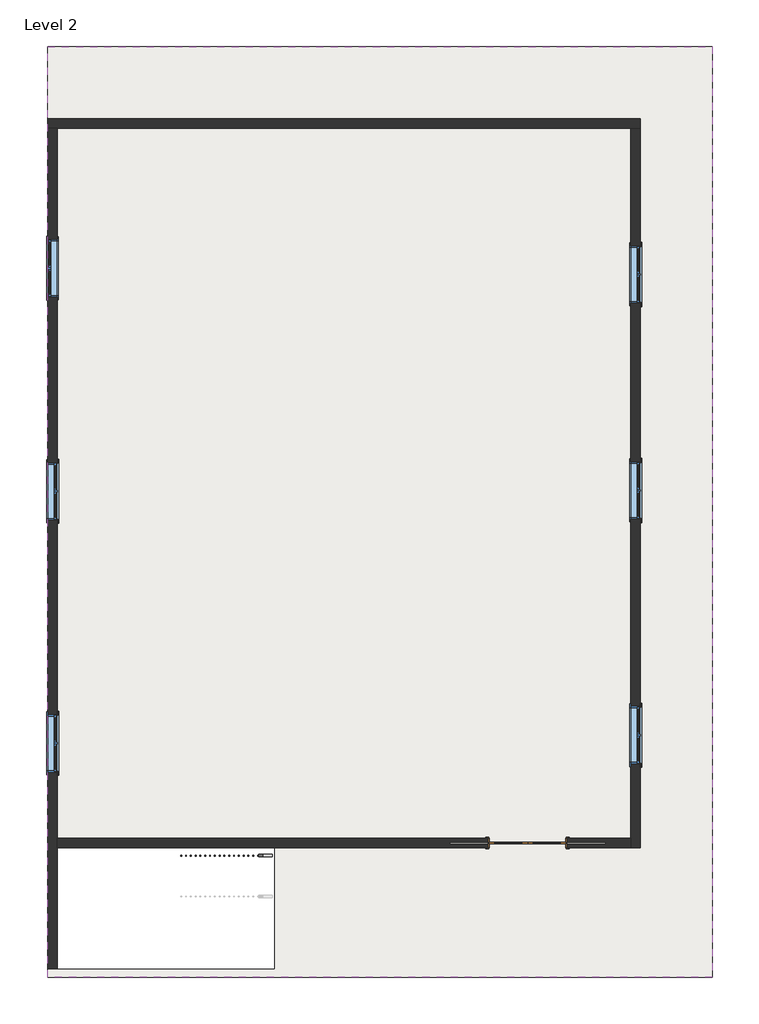
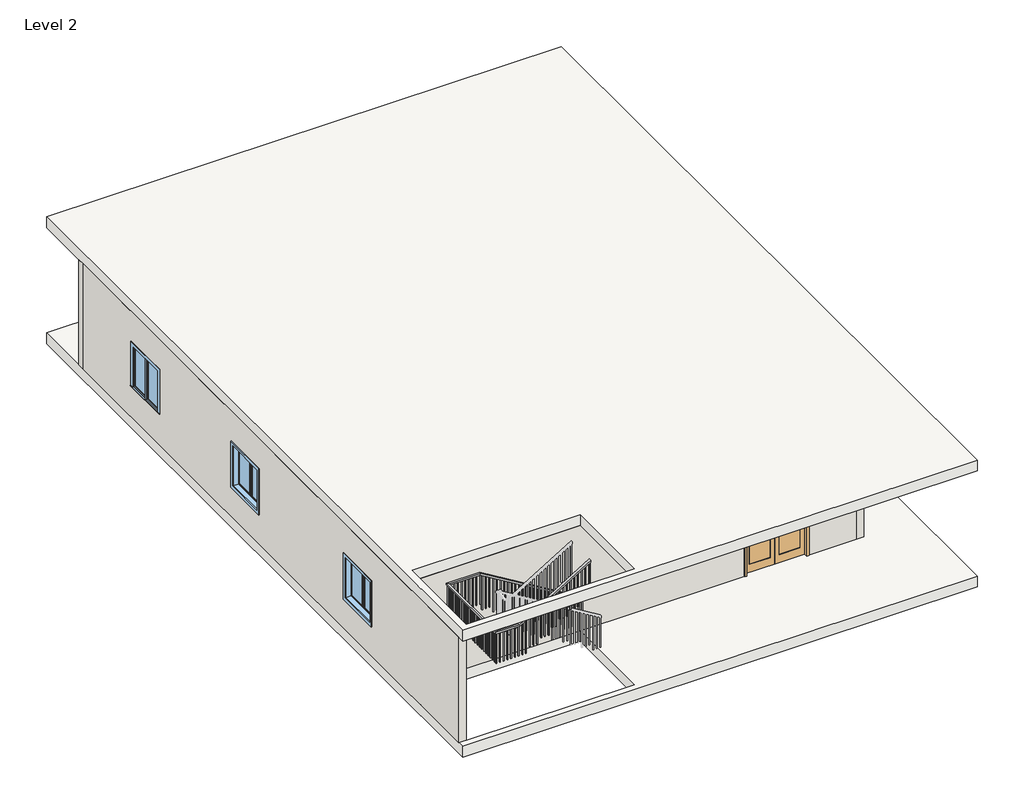
# One storey, part 1 of 2: 6 windows, 4 walls, 2 slabs, 1 door, 1 railing.
"""IFC4 building model written with IfcOpenShell, lengths in millimetres."""

from ifc_helpers import new_model, si_unit, frame, origin, place, context, project, spatial, polyline, outline, extrude, faceted_brep, transform, mapped, element, save
from components import door_18a53484, window_0862ab64

model = new_model("IFC4")

# Units and contexts
model_context = context("Model", 3, world=origin())
ifc_project = project(units=[si_unit("LENGTHUNIT", "METRE", prefix="MILLI")], contexts=[model_context])

# Site, building, storey
site = spatial("IfcSite", under=ifc_project)
building = spatial("IfcBuilding", under=site)
storey = spatial("IfcBuildingStorey", under=building, Name="Level 2", Elevation=3048.0)

# Door
placement = place(None, origin())
door_shape = door_18a53484(model_context)
element("IfcDoor", 1, ObjectType="Door-Interior-Double-Pocket-2_Panel-Wood : 64\" x 80\"", at=placement, inside=storey, context=model_context, shape_type="MappedRepresentation", body=[
    mapped(door_shape, transform((-1633.6127533, -5879.8242744, 3048.0), x_axis=(1.0, 0.0, 0.0), y_axis=(0.0, 1.0, 0.0), z_axis=(0.0, 0.0, 1.0))),
])

# Railing
element("IfcRailing", 2, ObjectType="Handrail - Rectangular", at=placement, inside=storey, context=model_context, shape_type="SolidModel", body=[
    faceted_brep([(-7036.5382419, -6171.9242744, 4131.7333333), (-7036.5382419, -6171.9242744, 4072.3318731), (-7036.5382419, -6121.1242744, 4072.3318731), (-7036.5382419, -6121.1242744, 4131.7333333), (-9830.5382419, -6171.9242744, 5825.0666667), (-9844.7306513, -6171.9242744, 5774.2666667), (-9844.7306513, -6121.1242744, 5774.2666667), (-9830.5382419, -6121.1242744, 5825.0666667), (-10694.1382419, -6171.9242744, 5825.0666667), (-10694.1382419, -6171.9242744, 5774.2666667), (-10744.9382419, -6121.1242744, 5774.2666667), (-10744.9382419, -6121.1242744, 5825.0666667), (-10694.1382419, -8420.4243151, 5825.0666667), (-10694.1382419, -8420.4243151, 5774.2666667), (-10744.9382419, -8471.2243151, 5774.2666667), (-10744.9382419, -8471.2243151, 5825.0666667), (-10109.9382419, -8420.4243151, 5825.0666667), (-10095.7458325, -8420.4243151, 5774.2666667), (-10095.7458325, -8471.2243151, 5774.2666667), (-10109.9382419, -8471.2243151, 5825.0666667), (-8154.1382419, -8420.4243151, 7010.4), (-8154.1382419, -8471.2243151, 7010.4), (-8154.1382419, -8471.2243151, 6950.9985397), (-8154.1382419, -8420.4243151, 6950.9985397)], [[[0, 1, 2, 3]], [[1, 0, 4, 5]], [[2, 1, 5, 6]], [[3, 2, 6, 7]], [[0, 3, 7, 4]], [[5, 4, 8, 9]], [[6, 5, 9, 10]], [[7, 6, 10, 11]], [[4, 7, 11, 8]], [[9, 8, 12, 13]], [[10, 9, 13, 14]], [[11, 10, 14, 15]], [[8, 11, 15, 12]], [[13, 12, 16, 17]], [[14, 13, 17, 18]], [[15, 14, 18, 19]], [[12, 15, 19, 16]], [[20, 21, 22, 23]], [[17, 16, 20, 23]], [[18, 17, 23, 22]], [[19, 18, 22, 21]], [[16, 19, 21, 20]]]),
    extrude(outline(polyline([(6941.3773276, -8170.0132419), (6929.8318731, -8189.0632419), (5926.6666667, -8189.0632419), (5926.6666667, -8170.0132419), (6941.3773276, -8170.0132419)])), frame((0.0, -8455.3493151, 0.0), z_axis=(0.0, 1.0, 0.0), x_axis=(0.0, 0.0, 1.0)), (0.0, 0.0, 1.0), 19.05),
    extrude(outline(polyline([(6879.80157, -8271.6132419), (6868.2561155, -8290.6632419), (5926.6666667, -8290.6632419), (5926.6666667, -8271.6132419), (6879.80157, -8271.6132419)])), frame((0.0, -8455.3493151, 0.0), z_axis=(0.0, 1.0, 0.0), x_axis=(0.0, 0.0, 1.0)), (0.0, 0.0, 1.0), 19.05),
    extrude(outline(polyline([(6818.2258125, -8373.2132419), (6806.6803579, -8392.2632419), (5926.6666667, -8392.2632419), (5926.6666667, -8373.2132419), (6818.2258125, -8373.2132419)])), frame((0.0, -8455.3493151, 0.0), z_axis=(0.0, 1.0, 0.0), x_axis=(0.0, 0.0, 1.0)), (0.0, 0.0, 1.0), 19.05),
    extrude(outline(polyline([(6756.6500549, -8474.8132419), (6745.1046004, -8493.8632419), (5757.3333333, -8493.8632419), (5757.3333333, -8474.8132419), (6756.6500549, -8474.8132419)])), frame((0.0, -8455.3493151, 0.0), z_axis=(0.0, 1.0, 0.0), x_axis=(0.0, 0.0, 1.0)), (0.0, 0.0, 1.0), 19.05),
    extrude(outline(polyline([(6695.0742973, -8576.4132419), (6683.5288428, -8595.4632419), (5757.3333333, -8595.4632419), (5757.3333333, -8576.4132419), (6695.0742973, -8576.4132419)])), frame((0.0, -8455.3493151, 0.0), z_axis=(0.0, 1.0, 0.0), x_axis=(0.0, 0.0, 1.0)), (0.0, 0.0, 1.0), 19.05),
    extrude(outline(polyline([(6633.4985397, -8678.0132419), (6621.9530852, -8697.0632419), (5757.3333333, -8697.0632419), (5757.3333333, -8678.0132419), (6633.4985397, -8678.0132419)])), frame((0.0, -8455.3493151, 0.0), z_axis=(0.0, 1.0, 0.0), x_axis=(0.0, 0.0, 1.0)), (0.0, 0.0, 1.0), 19.05),
    extrude(outline(polyline([(6571.9227822, -8779.6132419), (6560.3773276, -8798.6632419), (5588.0, -8798.6632419), (5588.0, -8779.6132419), (6571.9227822, -8779.6132419)])), frame((0.0, -8455.3493151, 0.0), z_axis=(0.0, 1.0, 0.0), x_axis=(0.0, 0.0, 1.0)), (0.0, 0.0, 1.0), 19.05),
    extrude(outline(polyline([(6510.3470246, -8881.2132419), (6498.80157, -8900.2632419), (5588.0, -8900.2632419), (5588.0, -8881.2132419), (6510.3470246, -8881.2132419)])), frame((0.0, -8455.3493151, 0.0), z_axis=(0.0, 1.0, 0.0), x_axis=(0.0, 0.0, 1.0)), (0.0, 0.0, 1.0), 19.05),
    extrude(outline(polyline([(6448.771267, -8982.8132419), (6437.2258125, -9001.8632419), (5588.0, -9001.8632419), (5588.0, -8982.8132419), (6448.771267, -8982.8132419)])), frame((0.0, -8455.3493151, 0.0), z_axis=(0.0, 1.0, 0.0), x_axis=(0.0, 0.0, 1.0)), (0.0, 0.0, 1.0), 19.05),
    extrude(outline(polyline([(6387.1955094, -9084.4132419), (6375.6500549, -9103.4632419), (5418.6666667, -9103.4632419), (5418.6666667, -9084.4132419), (6387.1955094, -9084.4132419)])), frame((0.0, -8455.3493151, 0.0), z_axis=(0.0, 1.0, 0.0), x_axis=(0.0, 0.0, 1.0)), (0.0, 0.0, 1.0), 19.05),
    extrude(outline(polyline([(6325.6197519, -9186.0132419), (6314.0742973, -9205.0632419), (5418.6666667, -9205.0632419), (5418.6666667, -9186.0132419), (6325.6197519, -9186.0132419)])), frame((0.0, -8455.3493151, 0.0), z_axis=(0.0, 1.0, 0.0), x_axis=(0.0, 0.0, 1.0)), (0.0, 0.0, 1.0), 19.05),
    extrude(outline(polyline([(6264.0439943, -9287.6132419), (6252.4985397, -9306.6632419), (5249.3333333, -9306.6632419), (5249.3333333, -9287.6132419), (6264.0439943, -9287.6132419)])), frame((0.0, -8455.3493151, 0.0), z_axis=(0.0, 1.0, 0.0), x_axis=(0.0, 0.0, 1.0)), (0.0, 0.0, 1.0), 19.05),
    extrude(outline(polyline([(6202.4682367, -9389.2132419), (6190.9227822, -9408.2632419), (5249.3333333, -9408.2632419), (5249.3333333, -9389.2132419), (6202.4682367, -9389.2132419)])), frame((0.0, -8455.3493151, 0.0), z_axis=(0.0, 1.0, 0.0), x_axis=(0.0, 0.0, 1.0)), (0.0, 0.0, 1.0), 19.05),
    extrude(outline(polyline([(6140.8924791, -9490.8132419), (6129.3470246, -9509.8632419), (5249.3333333, -9509.8632419), (5249.3333333, -9490.8132419), (6140.8924791, -9490.8132419)])), frame((0.0, -8455.3493151, 0.0), z_axis=(0.0, 1.0, 0.0), x_axis=(0.0, 0.0, 1.0)), (0.0, 0.0, 1.0), 19.05),
    extrude(outline(polyline([(6079.3167216, -9592.4132419), (6067.771267, -9611.4632419), (5080.0, -9611.4632419), (5080.0, -9592.4132419), (6079.3167216, -9592.4132419)])), frame((0.0, -8455.3493151, 0.0), z_axis=(0.0, 1.0, 0.0), x_axis=(0.0, 0.0, 1.0)), (0.0, 0.0, 1.0), 19.05),
    extrude(outline(polyline([(6017.740964, -9694.0132419), (6006.1955094, -9713.0632419), (5080.0, -9713.0632419), (5080.0, -9694.0132419), (6017.740964, -9694.0132419)])), frame((0.0, -8455.3493151, 0.0), z_axis=(0.0, 1.0, 0.0), x_axis=(0.0, 0.0, 1.0)), (0.0, 0.0, 1.0), 19.05),
    extrude(outline(polyline([(5956.1652064, -9795.6132419), (5944.6197519, -9814.6632419), (5080.0, -9814.6632419), (5080.0, -9795.6132419), (5956.1652064, -9795.6132419)])), frame((0.0, -8455.3493151, 0.0), z_axis=(0.0, 1.0, 0.0), x_axis=(0.0, 0.0, 1.0)), (0.0, 0.0, 1.0), 19.05),
    extrude(outline(polyline([(5894.5894488, -9897.2132419), (5883.0439943, -9916.2632419), (4910.6666667, -9916.2632419), (4910.6666667, -9897.2132419), (5894.5894488, -9897.2132419)])), frame((0.0, -8455.3493151, 0.0), z_axis=(0.0, 1.0, 0.0), x_axis=(0.0, 0.0, 1.0)), (0.0, 0.0, 1.0), 19.05),
    extrude(outline(polyline([(5833.0136913, -9998.8132419), (5821.4682367, -10017.8632419), (4910.6666667, -10017.8632419), (4910.6666667, -9998.8132419), (5833.0136913, -9998.8132419)])), frame((0.0, -8455.3493151, 0.0), z_axis=(0.0, 1.0, 0.0), x_axis=(0.0, 0.0, 1.0)), (0.0, 0.0, 1.0), 19.05),
    extrude(outline(polyline([(-10221.0632419, -8455.3493151), (-10221.0632419, -8436.2993151), (-10202.0132419, -8436.2993151), (-10202.0132419, -8455.3493151), (-10221.0632419, -8455.3493151)])), frame((0.0, 0.0, 4910.6666667), z_axis=(0.0, 0.0, 1.0), x_axis=(1.0, 0.0, 0.0)), (0.0, 0.0, 1.0), 863.6),
    extrude(outline(polyline([(-10322.6632419, -8455.3493151), (-10322.6632419, -8436.2993151), (-10303.6132419, -8436.2993151), (-10303.6132419, -8455.3493151), (-10322.6632419, -8455.3493151)])), frame((0.0, 0.0, 4910.6666667), z_axis=(0.0, 0.0, 1.0), x_axis=(1.0, 0.0, 0.0)), (0.0, 0.0, 1.0), 863.6),
    extrude(outline(polyline([(-10424.2632419, -8455.3493151), (-10424.2632419, -8436.2993151), (-10405.2132419, -8436.2993151), (-10405.2132419, -8455.3493151), (-10424.2632419, -8455.3493151)])), frame((0.0, 0.0, 4910.6666667), z_axis=(0.0, 0.0, 1.0), x_axis=(1.0, 0.0, 0.0)), (0.0, 0.0, 1.0), 863.6),
    extrude(outline(polyline([(-10525.8632419, -8455.3493151), (-10525.8632419, -8436.2993151), (-10506.8132419, -8436.2993151), (-10506.8132419, -8455.3493151), (-10525.8632419, -8455.3493151)])), frame((0.0, 0.0, 4910.6666667), z_axis=(0.0, 0.0, 1.0), x_axis=(1.0, 0.0, 0.0)), (0.0, 0.0, 1.0), 863.6),
    extrude(outline(polyline([(-10627.4632419, -8455.3493151), (-10627.4632419, -8436.2993151), (-10608.4132419, -8436.2993151), (-10608.4132419, -8455.3493151), (-10627.4632419, -8455.3493151)])), frame((0.0, 0.0, 4910.6666667), z_axis=(0.0, 0.0, 1.0), x_axis=(1.0, 0.0, 0.0)), (0.0, 0.0, 1.0), 863.6),
    extrude(outline(polyline([(-10729.0632419, -8372.1992744), (-10710.0132419, -8372.1992744), (-10710.0132419, -8391.2492744), (-10729.0632419, -8391.2492744), (-10729.0632419, -8372.1992744)])), frame((0.0, 0.0, 4910.6666667), z_axis=(0.0, 0.0, 1.0), x_axis=(1.0, 0.0, 0.0)), (0.0, 0.0, 1.0), 863.6),
    extrude(outline(polyline([(-10729.0632419, -8270.5992744), (-10710.0132419, -8270.5992744), (-10710.0132419, -8289.6492744), (-10729.0632419, -8289.6492744), (-10729.0632419, -8270.5992744)])), frame((0.0, 0.0, 4910.6666667), z_axis=(0.0, 0.0, 1.0), x_axis=(1.0, 0.0, 0.0)), (0.0, 0.0, 1.0), 863.6),
    extrude(outline(polyline([(-10729.0632419, -8168.9992744), (-10710.0132419, -8168.9992744), (-10710.0132419, -8188.0492744), (-10729.0632419, -8188.0492744), (-10729.0632419, -8168.9992744)])), frame((0.0, 0.0, 4910.6666667), z_axis=(0.0, 0.0, 1.0), x_axis=(1.0, 0.0, 0.0)), (0.0, 0.0, 1.0), 863.6),
    extrude(outline(polyline([(-10729.0632419, -8067.3992744), (-10710.0132419, -8067.3992744), (-10710.0132419, -8086.4492744), (-10729.0632419, -8086.4492744), (-10729.0632419, -8067.3992744)])), frame((0.0, 0.0, 4910.6666667), z_axis=(0.0, 0.0, 1.0), x_axis=(1.0, 0.0, 0.0)), (0.0, 0.0, 1.0), 863.6),
    extrude(outline(polyline([(-10729.0632419, -7965.7992744), (-10710.0132419, -7965.7992744), (-10710.0132419, -7984.8492744), (-10729.0632419, -7984.8492744), (-10729.0632419, -7965.7992744)])), frame((0.0, 0.0, 4910.6666667), z_axis=(0.0, 0.0, 1.0), x_axis=(1.0, 0.0, 0.0)), (0.0, 0.0, 1.0), 863.6),
    extrude(outline(polyline([(-10729.0632419, -7864.1992744), (-10710.0132419, -7864.1992744), (-10710.0132419, -7883.2492744), (-10729.0632419, -7883.2492744), (-10729.0632419, -7864.1992744)])), frame((0.0, 0.0, 4910.6666667), z_axis=(0.0, 0.0, 1.0), x_axis=(1.0, 0.0, 0.0)), (0.0, 0.0, 1.0), 863.6),
    extrude(outline(polyline([(-10729.0632419, -7762.5992744), (-10710.0132419, -7762.5992744), (-10710.0132419, -7781.6492744), (-10729.0632419, -7781.6492744), (-10729.0632419, -7762.5992744)])), frame((0.0, 0.0, 4910.6666667), z_axis=(0.0, 0.0, 1.0), x_axis=(1.0, 0.0, 0.0)), (0.0, 0.0, 1.0), 863.6),
    extrude(outline(polyline([(-10729.0632419, -7660.9992744), (-10710.0132419, -7660.9992744), (-10710.0132419, -7680.0492744), (-10729.0632419, -7680.0492744), (-10729.0632419, -7660.9992744)])), frame((0.0, 0.0, 4910.6666667), z_axis=(0.0, 0.0, 1.0), x_axis=(1.0, 0.0, 0.0)), (0.0, 0.0, 1.0), 863.6),
    extrude(outline(polyline([(-10729.0632419, -7559.3992744), (-10710.0132419, -7559.3992744), (-10710.0132419, -7578.4492744), (-10729.0632419, -7578.4492744), (-10729.0632419, -7559.3992744)])), frame((0.0, 0.0, 4910.6666667), z_axis=(0.0, 0.0, 1.0), x_axis=(1.0, 0.0, 0.0)), (0.0, 0.0, 1.0), 863.6),
    extrude(outline(polyline([(-10729.0632419, -7457.7992744), (-10710.0132419, -7457.7992744), (-10710.0132419, -7476.8492744), (-10729.0632419, -7476.8492744), (-10729.0632419, -7457.7992744)])), frame((0.0, 0.0, 4910.6666667), z_axis=(0.0, 0.0, 1.0), x_axis=(1.0, 0.0, 0.0)), (0.0, 0.0, 1.0), 863.6),
    extrude(outline(polyline([(-10729.0632419, -7356.1992744), (-10710.0132419, -7356.1992744), (-10710.0132419, -7375.2492744), (-10729.0632419, -7375.2492744), (-10729.0632419, -7356.1992744)])), frame((0.0, 0.0, 4910.6666667), z_axis=(0.0, 0.0, 1.0), x_axis=(1.0, 0.0, 0.0)), (0.0, 0.0, 1.0), 863.6),
    extrude(outline(polyline([(-10729.0632419, -7254.5992744), (-10710.0132419, -7254.5992744), (-10710.0132419, -7273.6492744), (-10729.0632419, -7273.6492744), (-10729.0632419, -7254.5992744)])), frame((0.0, 0.0, 4910.6666667), z_axis=(0.0, 0.0, 1.0), x_axis=(1.0, 0.0, 0.0)), (0.0, 0.0, 1.0), 863.6),
    extrude(outline(polyline([(-10729.0632419, -7152.9992744), (-10710.0132419, -7152.9992744), (-10710.0132419, -7172.0492744), (-10729.0632419, -7172.0492744), (-10729.0632419, -7152.9992744)])), frame((0.0, 0.0, 4910.6666667), z_axis=(0.0, 0.0, 1.0), x_axis=(1.0, 0.0, 0.0)), (0.0, 0.0, 1.0), 863.6),
    extrude(outline(polyline([(-10729.0632419, -7051.3992744), (-10710.0132419, -7051.3992744), (-10710.0132419, -7070.4492744), (-10729.0632419, -7070.4492744), (-10729.0632419, -7051.3992744)])), frame((0.0, 0.0, 4910.6666667), z_axis=(0.0, 0.0, 1.0), x_axis=(1.0, 0.0, 0.0)), (0.0, 0.0, 1.0), 863.6),
    extrude(outline(polyline([(-10729.0632419, -6949.7992744), (-10710.0132419, -6949.7992744), (-10710.0132419, -6968.8492744), (-10729.0632419, -6968.8492744), (-10729.0632419, -6949.7992744)])), frame((0.0, 0.0, 4910.6666667), z_axis=(0.0, 0.0, 1.0), x_axis=(1.0, 0.0, 0.0)), (0.0, 0.0, 1.0), 863.6),
    extrude(outline(polyline([(-10729.0632419, -6848.1992744), (-10710.0132419, -6848.1992744), (-10710.0132419, -6867.2492744), (-10729.0632419, -6867.2492744), (-10729.0632419, -6848.1992744)])), frame((0.0, 0.0, 4910.6666667), z_axis=(0.0, 0.0, 1.0), x_axis=(1.0, 0.0, 0.0)), (0.0, 0.0, 1.0), 863.6),
    extrude(outline(polyline([(-10729.0632419, -6746.5992744), (-10710.0132419, -6746.5992744), (-10710.0132419, -6765.6492744), (-10729.0632419, -6765.6492744), (-10729.0632419, -6746.5992744)])), frame((0.0, 0.0, 4910.6666667), z_axis=(0.0, 0.0, 1.0), x_axis=(1.0, 0.0, 0.0)), (0.0, 0.0, 1.0), 863.6),
    extrude(outline(polyline([(-10729.0632419, -6644.9992744), (-10710.0132419, -6644.9992744), (-10710.0132419, -6664.0492744), (-10729.0632419, -6664.0492744), (-10729.0632419, -6644.9992744)])), frame((0.0, 0.0, 4910.6666667), z_axis=(0.0, 0.0, 1.0), x_axis=(1.0, 0.0, 0.0)), (0.0, 0.0, 1.0), 863.6),
    extrude(outline(polyline([(-10729.0632419, -6543.3992744), (-10710.0132419, -6543.3992744), (-10710.0132419, -6562.4492744), (-10729.0632419, -6562.4492744), (-10729.0632419, -6543.3992744)])), frame((0.0, 0.0, 4910.6666667), z_axis=(0.0, 0.0, 1.0), x_axis=(1.0, 0.0, 0.0)), (0.0, 0.0, 1.0), 863.6),
    extrude(outline(polyline([(-10729.0632419, -6441.7992744), (-10710.0132419, -6441.7992744), (-10710.0132419, -6460.8492744), (-10729.0632419, -6460.8492744), (-10729.0632419, -6441.7992744)])), frame((0.0, 0.0, 4910.6666667), z_axis=(0.0, 0.0, 1.0), x_axis=(1.0, 0.0, 0.0)), (0.0, 0.0, 1.0), 863.6),
    extrude(outline(polyline([(-10729.0632419, -6340.1992744), (-10710.0132419, -6340.1992744), (-10710.0132419, -6359.2492744), (-10729.0632419, -6359.2492744), (-10729.0632419, -6340.1992744)])), frame((0.0, 0.0, 4910.6666667), z_axis=(0.0, 0.0, 1.0), x_axis=(1.0, 0.0, 0.0)), (0.0, 0.0, 1.0), 863.6),
    extrude(outline(polyline([(-10729.0632419, -6238.5992744), (-10710.0132419, -6238.5992744), (-10710.0132419, -6257.6492744), (-10729.0632419, -6257.6492744), (-10729.0632419, -6238.5992744)])), frame((0.0, 0.0, 4910.6666667), z_axis=(0.0, 0.0, 1.0), x_axis=(1.0, 0.0, 0.0)), (0.0, 0.0, 1.0), 863.6),
    extrude(outline(polyline([(-10633.8132419, -6136.9992744), (-10633.8132419, -6156.0492744), (-10652.8632419, -6156.0492744), (-10652.8632419, -6136.9992744), (-10633.8132419, -6136.9992744)])), frame((0.0, 0.0, 4910.6666667), z_axis=(0.0, 0.0, 1.0), x_axis=(1.0, 0.0, 0.0)), (0.0, 0.0, 1.0), 863.6),
    extrude(outline(polyline([(-10532.2132419, -6136.9992744), (-10532.2132419, -6156.0492744), (-10551.2632419, -6156.0492744), (-10551.2632419, -6136.9992744), (-10532.2132419, -6136.9992744)])), frame((0.0, 0.0, 4910.6666667), z_axis=(0.0, 0.0, 1.0), x_axis=(1.0, 0.0, 0.0)), (0.0, 0.0, 1.0), 863.6),
    extrude(outline(polyline([(-10430.6132419, -6136.9992744), (-10430.6132419, -6156.0492744), (-10449.6632419, -6156.0492744), (-10449.6632419, -6136.9992744), (-10430.6132419, -6136.9992744)])), frame((0.0, 0.0, 4910.6666667), z_axis=(0.0, 0.0, 1.0), x_axis=(1.0, 0.0, 0.0)), (0.0, 0.0, 1.0), 863.6),
    extrude(outline(polyline([(-10329.0132419, -6136.9992744), (-10329.0132419, -6156.0492744), (-10348.0632419, -6156.0492744), (-10348.0632419, -6136.9992744), (-10329.0132419, -6136.9992744)])), frame((0.0, 0.0, 4910.6666667), z_axis=(0.0, 0.0, 1.0), x_axis=(1.0, 0.0, 0.0)), (0.0, 0.0, 1.0), 863.6),
    extrude(outline(polyline([(-10227.4132419, -6136.9992744), (-10227.4132419, -6156.0492744), (-10246.4632419, -6156.0492744), (-10246.4632419, -6136.9992744), (-10227.4132419, -6136.9992744)])), frame((0.0, 0.0, 4910.6666667), z_axis=(0.0, 0.0, 1.0), x_axis=(1.0, 0.0, 0.0)), (0.0, 0.0, 1.0), 863.6),
    extrude(outline(polyline([(-10125.8132419, -6136.9992744), (-10125.8132419, -6156.0492744), (-10144.8632419, -6156.0492744), (-10144.8632419, -6136.9992744), (-10125.8132419, -6136.9992744)])), frame((0.0, 0.0, 4910.6666667), z_axis=(0.0, 0.0, 1.0), x_axis=(1.0, 0.0, 0.0)), (0.0, 0.0, 1.0), 863.6),
    extrude(outline(polyline([(-10024.2132419, -6136.9992744), (-10024.2132419, -6156.0492744), (-10043.2632419, -6156.0492744), (-10043.2632419, -6136.9992744), (-10024.2132419, -6136.9992744)])), frame((0.0, 0.0, 4910.6666667), z_axis=(0.0, 0.0, 1.0), x_axis=(1.0, 0.0, 0.0)), (0.0, 0.0, 1.0), 863.6),
    extrude(outline(polyline([(-9922.6132419, -6136.9992744), (-9922.6132419, -6156.0492744), (-9941.6632419, -6156.0492744), (-9941.6632419, -6136.9992744), (-9922.6132419, -6136.9992744)])), frame((0.0, 0.0, 4910.6666667), z_axis=(0.0, 0.0, 1.0), x_axis=(1.0, 0.0, 0.0)), (0.0, 0.0, 1.0), 863.6),
    extrude(outline(polyline([(5729.1046004, -9770.2132419), (5740.6500549, -9789.2632419), (4741.3333333, -9789.2632419), (4741.3333333, -9770.2132419), (5729.1046004, -9770.2132419)])), frame((0.0, -6156.0492744, 0.0), z_axis=(0.0, 1.0, 0.0), x_axis=(0.0, 0.0, 1.0)), (0.0, 0.0, 1.0), 19.05),
    extrude(outline(polyline([(5667.5288428, -9668.6132419), (5679.0742973, -9687.6632419), (4741.3333333, -9687.6632419), (4741.3333333, -9668.6132419), (5667.5288428, -9668.6132419)])), frame((0.0, -6156.0492744, 0.0), z_axis=(0.0, 1.0, 0.0), x_axis=(0.0, 0.0, 1.0)), (0.0, 0.0, 1.0), 19.05),
    extrude(outline(polyline([(5605.9530852, -9567.0132419), (5617.4985397, -9586.0632419), (4741.3333333, -9586.0632419), (4741.3333333, -9567.0132419), (5605.9530852, -9567.0132419)])), frame((0.0, -6156.0492744, 0.0), z_axis=(0.0, 1.0, 0.0), x_axis=(0.0, 0.0, 1.0)), (0.0, 0.0, 1.0), 19.05),
    extrude(outline(polyline([(5544.3773276, -9465.4132419), (5555.9227822, -9484.4632419), (4572.0, -9484.4632419), (4572.0, -9465.4132419), (5544.3773276, -9465.4132419)])), frame((0.0, -6156.0492744, 0.0), z_axis=(0.0, 1.0, 0.0), x_axis=(0.0, 0.0, 1.0)), (0.0, 0.0, 1.0), 19.05),
    extrude(outline(polyline([(5482.80157, -9363.8132419), (5494.3470246, -9382.8632419), (4572.0, -9382.8632419), (4572.0, -9363.8132419), (5482.80157, -9363.8132419)])), frame((0.0, -6156.0492744, 0.0), z_axis=(0.0, 1.0, 0.0), x_axis=(0.0, 0.0, 1.0)), (0.0, 0.0, 1.0), 19.05),
    extrude(outline(polyline([(5421.2258125, -9262.2132419), (5432.771267, -9281.2632419), (4572.0, -9281.2632419), (4572.0, -9262.2132419), (5421.2258125, -9262.2132419)])), frame((0.0, -6156.0492744, 0.0), z_axis=(0.0, 1.0, 0.0), x_axis=(0.0, 0.0, 1.0)), (0.0, 0.0, 1.0), 19.05),
    extrude(outline(polyline([(5359.6500549, -9160.6132419), (5371.1955094, -9179.6632419), (4402.6666667, -9179.6632419), (4402.6666667, -9160.6132419), (5359.6500549, -9160.6132419)])), frame((0.0, -6156.0492744, 0.0), z_axis=(0.0, 1.0, 0.0), x_axis=(0.0, 0.0, 1.0)), (0.0, 0.0, 1.0), 19.05),
    extrude(outline(polyline([(5298.0742973, -9059.0132419), (5309.6197519, -9078.0632419), (4402.6666667, -9078.0632419), (4402.6666667, -9059.0132419), (5298.0742973, -9059.0132419)])), frame((0.0, -6156.0492744, 0.0), z_axis=(0.0, 1.0, 0.0), x_axis=(0.0, 0.0, 1.0)), (0.0, 0.0, 1.0), 19.05),
    extrude(outline(polyline([(5236.4985397, -8957.4132419), (5248.0439943, -8976.4632419), (4233.3333333, -8976.4632419), (4233.3333333, -8957.4132419), (5236.4985397, -8957.4132419)])), frame((0.0, -6156.0492744, 0.0), z_axis=(0.0, 1.0, 0.0), x_axis=(0.0, 0.0, 1.0)), (0.0, 0.0, 1.0), 19.05),
    extrude(outline(polyline([(5174.9227822, -8855.8132419), (5186.4682367, -8874.8632419), (4233.3333333, -8874.8632419), (4233.3333333, -8855.8132419), (5174.9227822, -8855.8132419)])), frame((0.0, -6156.0492744, 0.0), z_axis=(0.0, 1.0, 0.0), x_axis=(0.0, 0.0, 1.0)), (0.0, 0.0, 1.0), 19.05),
    extrude(outline(polyline([(5113.3470246, -8754.2132419), (5124.8924791, -8773.2632419), (4233.3333333, -8773.2632419), (4233.3333333, -8754.2132419), (5113.3470246, -8754.2132419)])), frame((0.0, -6156.0492744, 0.0), z_axis=(0.0, 1.0, 0.0), x_axis=(0.0, 0.0, 1.0)), (0.0, 0.0, 1.0), 19.05),
    extrude(outline(polyline([(5051.771267, -8652.6132419), (5063.3167216, -8671.6632419), (4064.0, -8671.6632419), (4064.0, -8652.6132419), (5051.771267, -8652.6132419)])), frame((0.0, -6156.0492744, 0.0), z_axis=(0.0, 1.0, 0.0), x_axis=(0.0, 0.0, 1.0)), (0.0, 0.0, 1.0), 19.05),
    extrude(outline(polyline([(4990.1955094, -8551.0132419), (5001.740964, -8570.0632419), (4064.0, -8570.0632419), (4064.0, -8551.0132419), (4990.1955094, -8551.0132419)])), frame((0.0, -6156.0492744, 0.0), z_axis=(0.0, 1.0, 0.0), x_axis=(0.0, 0.0, 1.0)), (0.0, 0.0, 1.0), 19.05),
    extrude(outline(polyline([(4928.6197519, -8449.4132419), (4940.1652064, -8468.4632419), (4064.0, -8468.4632419), (4064.0, -8449.4132419), (4928.6197519, -8449.4132419)])), frame((0.0, -6156.0492744, 0.0), z_axis=(0.0, 1.0, 0.0), x_axis=(0.0, 0.0, 1.0)), (0.0, 0.0, 1.0), 19.05),
    extrude(outline(polyline([(4867.0439943, -8347.8132419), (4878.5894488, -8366.8632419), (3894.6666667, -8366.8632419), (3894.6666667, -8347.8132419), (4867.0439943, -8347.8132419)])), frame((0.0, -6156.0492744, 0.0), z_axis=(0.0, 1.0, 0.0), x_axis=(0.0, 0.0, 1.0)), (0.0, 0.0, 1.0), 19.05),
    extrude(outline(polyline([(4805.4682367, -8246.2132419), (4817.0136913, -8265.2632419), (3894.6666667, -8265.2632419), (3894.6666667, -8246.2132419), (4805.4682367, -8246.2132419)])), frame((0.0, -6156.0492744, 0.0), z_axis=(0.0, 1.0, 0.0), x_axis=(0.0, 0.0, 1.0)), (0.0, 0.0, 1.0), 19.05),
    extrude(outline(polyline([(4743.8924791, -8144.6132419), (4755.4379337, -8163.6632419), (3894.6666667, -8163.6632419), (3894.6666667, -8144.6132419), (4743.8924791, -8144.6132419)])), frame((0.0, -6156.0492744, 0.0), z_axis=(0.0, 1.0, 0.0), x_axis=(0.0, 0.0, 1.0)), (0.0, 0.0, 1.0), 19.05),
    extrude(outline(polyline([(4682.3167216, -8043.0132419), (4693.8621761, -8062.0632419), (3725.3333333, -8062.0632419), (3725.3333333, -8043.0132419), (4682.3167216, -8043.0132419)])), frame((0.0, -6156.0492744, 0.0), z_axis=(0.0, 1.0, 0.0), x_axis=(0.0, 0.0, 1.0)), (0.0, 0.0, 1.0), 19.05),
    extrude(outline(polyline([(4620.740964, -7941.4132419), (4632.2864185, -7960.4632419), (3725.3333333, -7960.4632419), (3725.3333333, -7941.4132419), (4620.740964, -7941.4132419)])), frame((0.0, -6156.0492744, 0.0), z_axis=(0.0, 1.0, 0.0), x_axis=(0.0, 0.0, 1.0)), (0.0, 0.0, 1.0), 19.05),
    extrude(outline(polyline([(4559.1652064, -7839.8132419), (4570.710661, -7858.8632419), (3556.0, -7858.8632419), (3556.0, -7839.8132419), (4559.1652064, -7839.8132419)])), frame((0.0, -6156.0492744, 0.0), z_axis=(0.0, 1.0, 0.0), x_axis=(0.0, 0.0, 1.0)), (0.0, 0.0, 1.0), 19.05),
    extrude(outline(polyline([(4497.5894488, -7738.2132419), (4509.1349034, -7757.2632419), (3556.0, -7757.2632419), (3556.0, -7738.2132419), (4497.5894488, -7738.2132419)])), frame((0.0, -6156.0492744, 0.0), z_axis=(0.0, 1.0, 0.0), x_axis=(0.0, 0.0, 1.0)), (0.0, 0.0, 1.0), 19.05),
    extrude(outline(polyline([(4436.0136913, -7636.6132419), (4447.5591458, -7655.6632419), (3556.0, -7655.6632419), (3556.0, -7636.6132419), (4436.0136913, -7636.6132419)])), frame((0.0, -6156.0492744, 0.0), z_axis=(0.0, 1.0, 0.0), x_axis=(0.0, 0.0, 1.0)), (0.0, 0.0, 1.0), 19.05),
    extrude(outline(polyline([(4374.4379337, -7535.0132419), (4385.9833882, -7554.0632419), (3386.6666667, -7554.0632419), (3386.6666667, -7535.0132419), (4374.4379337, -7535.0132419)])), frame((0.0, -6156.0492744, 0.0), z_axis=(0.0, 1.0, 0.0), x_axis=(0.0, 0.0, 1.0)), (0.0, 0.0, 1.0), 19.05),
    extrude(outline(polyline([(4312.8621761, -7433.4132419), (4324.4076307, -7452.4632419), (3386.6666667, -7452.4632419), (3386.6666667, -7433.4132419), (4312.8621761, -7433.4132419)])), frame((0.0, -6156.0492744, 0.0), z_axis=(0.0, 1.0, 0.0), x_axis=(0.0, 0.0, 1.0)), (0.0, 0.0, 1.0), 19.05),
    extrude(outline(polyline([(4251.2864185, -7331.8132419), (4262.8318731, -7350.8632419), (3386.6666667, -7350.8632419), (3386.6666667, -7331.8132419), (4251.2864185, -7331.8132419)])), frame((0.0, -6156.0492744, 0.0), z_axis=(0.0, 1.0, 0.0), x_axis=(0.0, 0.0, 1.0)), (0.0, 0.0, 1.0), 19.05),
    extrude(outline(polyline([(4189.710661, -7230.2132419), (4201.2561155, -7249.2632419), (3217.3333333, -7249.2632419), (3217.3333333, -7230.2132419), (4189.710661, -7230.2132419)])), frame((0.0, -6156.0492744, 0.0), z_axis=(0.0, 1.0, 0.0), x_axis=(0.0, 0.0, 1.0)), (0.0, 0.0, 1.0), 19.05),
    extrude(outline(polyline([(4128.1349034, -7128.6132419), (4139.6803579, -7147.6632419), (3217.3333333, -7147.6632419), (3217.3333333, -7128.6132419), (4128.1349034, -7128.6132419)])), frame((0.0, -6156.0492744, 0.0), z_axis=(0.0, 1.0, 0.0), x_axis=(0.0, 0.0, 1.0)), (0.0, 0.0, 1.0), 19.05),
    extrude(outline(polyline([(-10119.4632419, -8455.3493151), (-10119.4632419, -8436.2993151), (-10100.4132419, -8436.2993151), (-10100.4132419, -8455.3493151), (-10119.4632419, -8455.3493151)])), frame((0.0, 0.0, 4910.6666667), z_axis=(0.0, 0.0, 1.0), x_axis=(1.0, 0.0, 0.0)), (0.0, 0.0, 1.0), 863.6),
    extrude(outline(polyline([(-10729.0632419, -8436.2993151), (-10710.0132419, -8436.2993151), (-10710.0132419, -8455.3493151), (-10729.0632419, -8455.3493151), (-10729.0632419, -8436.2993151)])), frame((0.0, 0.0, 4910.6666667), z_axis=(0.0, 0.0, 1.0), x_axis=(1.0, 0.0, 0.0)), (0.0, 0.0, 1.0), 863.6),
    extrude(outline(polyline([(-10710.0132419, -6136.9992744), (-10710.0132419, -6156.0492744), (-10729.0632419, -6156.0492744), (-10729.0632419, -6136.9992744), (-10710.0132419, -6136.9992744)])), frame((0.0, 0.0, 4910.6666667), z_axis=(0.0, 0.0, 1.0), x_axis=(1.0, 0.0, 0.0)), (0.0, 0.0, 1.0), 863.6),
    extrude(outline(polyline([(5759.8924791, -9821.0132419), (5771.4379337, -9840.0632419), (4910.6666667, -9840.0632419), (4910.6666667, -9821.0132419), (5759.8924791, -9821.0132419)])), frame((0.0, -6156.0492744, 0.0), z_axis=(0.0, 1.0, 0.0), x_axis=(0.0, 0.0, 1.0)), (0.0, 0.0, 1.0), 19.05),
    extrude(outline(polyline([(6950.9985397, -8154.1382419), (6939.4530852, -8173.1882419), (5926.6666667, -8173.1882419), (5926.6666667, -8154.1382419), (6950.9985397, -8154.1382419)])), frame((0.0, -8455.3493151, 0.0), z_axis=(0.0, 1.0, 0.0), x_axis=(0.0, 0.0, 1.0)), (0.0, 0.0, 1.0), 19.05),
    extrude(outline(polyline([(4072.3318731, -7036.5382419), (4083.8773276, -7055.5882419), (3217.3333333, -7055.5882419), (3217.3333333, -7036.5382419), (4072.3318731, -7036.5382419)])), frame((0.0, -6156.0492744, 0.0), z_axis=(0.0, 1.0, 0.0), x_axis=(0.0, 0.0, 1.0)), (0.0, 0.0, 1.0), 19.05),
])

# Slabs
element("IfcSlab", 3, ObjectType="Generic - 12\"", at=placement, inside=storey, context=model_context, shape_type="SweptSolid", body=[
    extrude(outline(polyline([(-11793.6127533, 10985.7757256), (2277.9872467, 10985.7757256), (2277.9872467, -8724.6242744), (-11793.6127533, -8724.6242744), (-11793.6127533, 10985.7757256)]), holes=[polyline([(-6994.8503559, -5981.4242744), (-11590.4127533, -5981.4242744), (-11590.4127533, -8542.0083309), (-6994.8503559, -8542.0083309), (-6994.8503559, -5981.4242744)])]), frame((0.0, 0.0, 2743.2), z_axis=(0.0, 0.0, 1.0), x_axis=(1.0, 0.0, 0.0)), (0.0, 0.0, 1.0), 304.8),
])
element("IfcSlab", 4, ObjectType="Generic - 12\"", at=placement, inside=storey, context=model_context, shape_type="SweptSolid", body=[
    extrude(outline(polyline([(-11793.6127533, 10985.7757256), (2277.9872467, 10985.7757256), (2277.9872467, -8724.6242744), (-11793.6127533, -8724.6242744), (-11793.6127533, 10985.7757256)]), holes=[polyline([(-6994.8503559, -5981.4242744), (-11590.4127533, -5981.4242744), (-11590.4127533, -8542.0083309), (-6994.8503559, -8542.0083309), (-6994.8503559, -5981.4242744)])]), frame((0.0, 0.0, 6096.0), z_axis=(0.0, 0.0, 1.0), x_axis=(1.0, 0.0, 0.0)), (0.0, 0.0, 1.0), 304.8),
])

# Walls
element("IfcWall", 5, ObjectType="Generic - 8\"", at=placement, inside=storey, context=model_context, shape_type="Brep", body=[
    faceted_brep([(-11793.6127533, 9258.5757256, 3048.0), (-11590.4127533, 9258.5757256, 3048.0), (550.7872467, 9258.5757256, 3048.0), (753.9872467, 9258.5757256, 3048.0), (753.9872467, 9258.5757256, 6096.0), (550.7872467, 9258.5757256, 6096.0), (-11590.4127533, 9258.5757256, 6096.0), (-11793.6127533, 9258.5757256, 6096.0), (-11793.6127533, 9461.7757256, 3048.0), (-11793.6127533, 9461.7757256, 6096.0), (753.9872467, 9461.7757256, 6096.0), (753.9872467, 9461.7757256, 3048.0)], [[[0, 1, 2, 3, 4, 5, 6, 7]], [[8, 9, 10, 11]], [[3, 2, 1, 0, 8, 11]], [[7, 6, 5, 4, 10, 9]], [[4, 3, 11, 10]], [[0, 7, 9, 8]]]),
])
element("IfcWall", 6, ObjectType="Generic - 8\"", at=placement, inside=storey, context=model_context, shape_type="Brep", body=[
    faceted_brep([(550.7872467, 9258.5757256, 3048.0), (550.7872467, -5778.2242744, 3048.0), (550.7872467, -5981.4242744, 3048.0), (550.7872467, -5981.4242744, 6096.0), (550.7872467, -5778.2242744, 6096.0), (550.7872467, 9258.5757256, 6096.0), (550.7872467, -4203.4242744, 5181.6), (550.7872467, -4203.4242744, 3962.4), (550.7872467, -2984.2242744, 3962.4), (550.7872467, -2984.2242744, 5181.6), (550.7872467, 978.1757256, 5181.6), (550.7872467, 978.1757256, 3962.4), (550.7872467, 2197.3757256, 3962.4), (550.7872467, 2197.3757256, 5181.6), (550.7872467, 5550.1757256, 5181.6), (550.7872467, 5550.1757256, 3962.4), (550.7872467, 6769.3757256, 3962.4), (550.7872467, 6769.3757256, 5181.6), (753.9872467, 9258.5757256, 3048.0), (753.9872467, 9258.5757256, 6096.0), (753.9872467, -5981.4242744, 6096.0), (753.9872467, -5981.4242744, 3048.0), (753.9872467, -4203.4242744, 5181.6), (753.9872467, -2984.2242744, 5181.6), (753.9872467, -2984.2242744, 3962.4), (753.9872467, -4203.4242744, 3962.4), (753.9872467, 978.1757256, 5181.6), (753.9872467, 2197.3757256, 5181.6), (753.9872467, 2197.3757256, 3962.4), (753.9872467, 978.1757256, 3962.4), (753.9872467, 5550.1757256, 5181.6), (753.9872467, 6769.3757256, 5181.6), (753.9872467, 6769.3757256, 3962.4), (753.9872467, 5550.1757256, 3962.4)], [[[0, 1, 2, 3, 4, 5], [6, 7, 8, 9], [10, 11, 12, 13], [14, 15, 16, 17]], [[18, 19, 20, 21], [22, 23, 24, 25], [26, 27, 28, 29], [30, 31, 32, 33]], [[2, 1, 0, 18, 21]], [[5, 4, 3, 20, 19]], [[0, 5, 19, 18]], [[3, 2, 21, 20]], [[7, 6, 22, 25]], [[8, 7, 25, 24]], [[9, 8, 24, 23]], [[6, 9, 23, 22]], [[11, 10, 26, 29]], [[12, 11, 29, 28]], [[13, 12, 28, 27]], [[10, 13, 27, 26]], [[15, 14, 30, 33]], [[16, 15, 33, 32]], [[17, 16, 32, 31]], [[14, 17, 31, 30]]]),
])
element("IfcWall", 7, ObjectType="Generic - 8\"", at=placement, inside=storey, context=model_context, shape_type="Brep", body=[
    faceted_brep([(-11590.4127533, -5778.2242744, 6096.0), (550.7872467, -5778.2242744, 6096.0), (550.7872467, -5778.2242744, 3048.0), (-795.4127533, -5778.2242744, 3048.0), (-795.4127533, -5778.2242744, 5105.4), (-2471.8127533, -5778.2242744, 5105.4), (-2471.8127533, -5778.2242744, 3048.0), (-11590.4127533, -5778.2242744, 3048.0), (550.7872467, -5981.4242744, 6096.0), (-11590.4127533, -5981.4242744, 6096.0), (-11590.4127533, -5981.4242744, 3048.0), (-2471.8127533, -5981.4242744, 3048.0), (-2471.8127533, -5981.4242744, 5105.4), (-795.4127533, -5981.4242744, 5105.4), (-795.4127533, -5981.4242744, 3048.0), (550.7872467, -5981.4242744, 3048.0), (-795.4127533, -5900.4617744, 3048.0), (17.3872467, -5900.4617744, 3048.0), (17.3872467, -5859.1867744, 3048.0), (-795.4127533, -5859.1867744, 3048.0), (-2471.8127533, -5859.1867744, 3048.0), (-3284.6127533, -5859.1867744, 3048.0), (-3284.6127533, -5900.4617744, 3048.0), (-2471.8127533, -5900.4617744, 3048.0), (17.3872467, -5859.1867744, 5105.4), (17.3872467, -5900.4617744, 5105.4), (-795.4127533, -5900.4617744, 5105.4), (-2471.8127533, -5900.4617744, 5105.4), (-3284.6127533, -5900.4617744, 5105.4), (-3284.6127533, -5859.1867744, 5105.4), (-2471.8127533, -5859.1867744, 5105.4), (-795.4127533, -5859.1867744, 5105.4)], [[[0, 1, 2, 3, 4, 5, 6, 7]], [[8, 9, 10, 11, 12, 13, 14, 15]], [[2, 15, 14, 16, 17, 18, 19, 3]], [[10, 7, 6, 20, 21, 22, 23, 11]], [[1, 0, 9, 8]], [[2, 1, 8, 15]], [[0, 7, 10, 9]], [[24, 25, 26, 13, 12, 27, 28, 29, 30, 5, 4, 31]], [[24, 31, 19, 18]], [[31, 4, 3, 19]], [[5, 30, 20, 6]], [[30, 29, 21, 20]], [[29, 28, 22, 21]], [[28, 27, 23, 22]], [[27, 12, 11, 23]], [[13, 26, 16, 14]], [[26, 25, 17, 16]], [[25, 24, 18, 17]]]),
])
element("IfcWall", 8, ObjectType="Generic - 8\"", at=placement, inside=storey, context=model_context, shape_type="Brep", body=[
    faceted_brep([(-11590.4127533, -8542.0083309, 3048.0), (-11590.4127533, -5981.4242744, 3048.0), (-11590.4127533, -5778.2242744, 3048.0), (-11590.4127533, 9258.5757256, 3048.0), (-11590.4127533, 9258.5757256, 6096.0), (-11590.4127533, -5778.2242744, 6096.0), (-11590.4127533, -5981.4242744, 6096.0), (-11590.4127533, -8542.0083309, 6096.0), (-11590.4127533, 6901.1916691, 5181.6), (-11590.4127533, 6901.1916691, 3962.4), (-11590.4127533, 5681.9916691, 3962.4), (-11590.4127533, 5681.9916691, 5181.6), (-11590.4127533, 957.5916691, 5181.6), (-11590.4127533, 2176.7916691, 5181.6), (-11590.4127533, 2176.7916691, 3962.4), (-11590.4127533, 957.5916691, 3962.4), (-11590.4127533, -4376.4083309, 5181.6), (-11590.4127533, -3157.2083309, 5181.6), (-11590.4127533, -3157.2083309, 3962.4), (-11590.4127533, -4376.4083309, 3962.4), (-11793.6127533, -8542.0083309, 3048.0), (-11793.6127533, -8542.0083309, 6096.0), (-11793.6127533, 9258.5757256, 6096.0), (-11793.6127533, 9258.5757256, 3048.0), (-11793.6127533, 6901.1916691, 5181.6), (-11793.6127533, 5681.9916691, 5181.6), (-11793.6127533, 5681.9916691, 3962.4), (-11793.6127533, 6901.1916691, 3962.4), (-11793.6127533, 957.5916691, 5181.6), (-11793.6127533, 957.5916691, 3962.4), (-11793.6127533, 2176.7916691, 3962.4), (-11793.6127533, 2176.7916691, 5181.6), (-11793.6127533, -4376.4083309, 5181.6), (-11793.6127533, -4376.4083309, 3962.4), (-11793.6127533, -3157.2083309, 3962.4), (-11793.6127533, -3157.2083309, 5181.6)], [[[0, 1, 2, 3, 4, 5, 6, 7], [8, 9, 10, 11], [12, 13, 14, 15], [16, 17, 18, 19]], [[20, 21, 22, 23], [24, 25, 26, 27], [28, 29, 30, 31], [32, 33, 34, 35]], [[3, 2, 1, 0, 20, 23]], [[7, 6, 5, 4, 22, 21]], [[0, 7, 21, 20]], [[4, 3, 23, 22]], [[9, 8, 24, 27]], [[10, 9, 27, 26]], [[11, 10, 26, 25]], [[8, 11, 25, 24]], [[29, 28, 12, 15]], [[30, 29, 15, 14]], [[31, 30, 14, 13]], [[28, 31, 13, 12]], [[33, 32, 16, 19]], [[34, 33, 19, 18]], [[35, 34, 18, 17]], [[32, 35, 17, 16]]]),
])

# Windows
window_shape = window_0862ab64(model_context)
element("IfcWindow", 9, ObjectType="Casement Dbl with Trim : 48\" x 48\"", at=placement, inside=storey, context=model_context, shape_type="MappedRepresentation", body=[
    mapped(window_shape, transform((633.3372467, -3593.8242744, 3048.0), x_axis=(0.0, -1.0, 0.0), y_axis=(1.0, 0.0, 0.0), z_axis=(0.0, 0.0, 1.0))),
])
element("IfcWindow", 10, ObjectType="Casement Dbl with Trim : 48\" x 48\"", at=placement, inside=storey, context=model_context, shape_type="MappedRepresentation", body=[
    mapped(window_shape, transform((633.3372467, 1587.7757256, 3048.0), x_axis=(0.0, -1.0, 0.0), y_axis=(1.0, 0.0, 0.0), z_axis=(0.0, 0.0, 1.0))),
])
element("IfcWindow", 11, ObjectType="Casement Dbl with Trim : 48\" x 48\"", at=placement, inside=storey, context=model_context, shape_type="MappedRepresentation", body=[
    mapped(window_shape, transform((633.3372467, 6159.7757256, 3048.0), x_axis=(0.0, -1.0, 0.0), y_axis=(1.0, 0.0, 0.0), z_axis=(0.0, 0.0, 1.0))),
])
element("IfcWindow", 12, ObjectType="Casement Dbl with Trim : 48\" x 48\"", at=placement, inside=storey, context=model_context, shape_type="MappedRepresentation", body=[
    mapped(window_shape, transform((-11672.9627533, 6291.5916691, 3048.0), x_axis=(0.0, 1.0, 0.0), y_axis=(-1.0, 0.0, 0.0), z_axis=(0.0, 0.0, 1.0))),
])
element("IfcWindow", 13, ObjectType="Casement Dbl with Trim : 48\" x 48\"", at=placement, inside=storey, context=model_context, shape_type="MappedRepresentation", body=[
    mapped(window_shape, transform((-11711.0627533, 1567.1916691, 3048.0), x_axis=(0.0, -1.0, 0.0), y_axis=(1.0, 0.0, 0.0), z_axis=(0.0, 0.0, 1.0))),
])
element("IfcWindow", 14, ObjectType="Casement Dbl with Trim : 48\" x 48\"", at=placement, inside=storey, context=model_context, shape_type="MappedRepresentation", body=[
    mapped(window_shape, transform((-11711.0627533, -3766.8083309, 3048.0), x_axis=(0.0, -1.0, 0.0), y_axis=(1.0, 0.0, 0.0), z_axis=(0.0, 0.0, 1.0))),
])

save(model, "model.ifc")

# Revit data of these elements
# Type "Door-Interior-Double-Pocket-2_Panel-Wood : 64\" x 80\""
#   Type Mark = "8"
#   Assembly Code = "C1020300"
#   Analytic Construction = "Wooden"
#   Top Rail = 0' - 4 11/16"
#   Thickness = 0' - 1 3/8"
#   Thermal Resistance (R) = 2.5876 (h·ft²·°F)/BTU
#   Stiles = 0' - 4 3/4"
#   Rough Width = 10' - 10"
#   Rough Height = 7' - 0 1/2"
#   Panel Width = 2' - 8"
#   Lock Rail = 0' - 7 1/2"
#   Location [instance default] = 2' - 9"
#   Height = 6' - 8"
#   Width = 5' - 4"
#   Heat Transfer Coefficient (U) = 0.3865 BTU/(h·ft²·°F)
#   Bottom Rail = 0' - 9 1/8"
#   Panel Open [instance default] = no
#   Trim Material = Cherry
#   Panel Material = Cherry
#   Frame Material = Cherry
#   Visual Light Transmittance = 0
#   Solar Heat Gain Coefficient = 0
#   Wall Closure = (empty or 0)
#   Function = (empty or 0)
# Type "Handrail - Rectangular"
#   Assembly Code = "C2010400"
#   built-in parameter 1008612 = 0.0416667 (stored number, unit not read)
#   built-in parameter 1008611 = 0.0416667 (stored number, unit not read)
#   built-in parameter 1008609 = 0.333333 (stored number, unit not read)
#   built-in parameter 1008604 = 0.166667 (stored number, unit not read)
#   built-in parameter 1008603 = 0.166667 (stored number, unit not read)
#   Railing Height = 3' - 0"
#   built-in parameter 1008630 = 2
#   built-in parameter 1008610 = 2
#   built-in parameter 1008618 = Baluster - Square : 3/4"
# Type "Generic - 12\""
#   Assembly Code = "B1010"
#   Function = 0
#   Layers, outside or top first: 1' - 0" no material (function 1)
# Type "Generic - 8\""
#   Assembly Code = "B2010"
#   Layers, outside or top first: 0' - 8" no material (function 1)
# Type "Casement Dbl with Trim : 48\" x 48\""
#   Type Mark = "10"
#   Construction Type Id = "GSP4R"
#   Assembly Code = "B2020100"
#   Analytic Construction = "1/8 in Pilkington single glazing"
#   Visual Light Transmittance = 0.9
#   Solar Heat Gain Coefficient = 0.78
#   Heat Transfer Coefficient (U) = 0.6496 BTU/(h·ft²·°F)
#   Height = 4' - 0"
#   Default Sill Height = 3' - 0"
#   Trim Projection - Ext. = 0' - 0 1/2"
#   Trim Projection - Int. = 0' - 0 3/4"
#   Trim Width - Exterior = 0' - 3 1/2"
#   Trim Width - Interior = 0' - 3 1/2"
#   Width = 4' - 0"
#   Window Inset = 0' - 0 3/4"
#   Define Thermal Properties by = 1
#   Glass Pane Material = Glass
#   Sash Material = Sash
#   Trim Exterior Material = Trim
#   Trim Interior Material = Trim
#   Wall Closure = (empty or 0)
# Element 1 (IfcDoor, "Door-Interior-Double-Pocket-2_Panel-Wood : 64\" x 80\"")
#   Location = 2' - 9"
#   Panel Open = no
#   Phase Created = New Construction
#   Materials on its faces: "Cherry"
# Element 2 (IfcRailing, "Handrail - Rectangular")
#   Phase Created = New Construction
# Element 3 (IfcSlab, "Generic - 12\"")
#   built-in parameter 1001955 = 1.5708 (stored number, unit not read)
#   Height Offset From Level = 0' - 0"
#   Phase Created = New Construction
#   Materials on its faces: "Default Floor"
# Element 4 (IfcSlab, "Generic - 12\"")
#   built-in parameter 1001955 = 1.5708 (stored number, unit not read)
#   Height Offset From Level = 11' - 0"
#   Phase Created = New Construction
#   Materials on its faces: "Default Floor"
# Elements 5, 6, 7, 8 (IfcWall, "Generic - 8\"")
#   Top Offset = 0' - 0"
#   Base Offset = 0' - 0"
#   Unconnected Height = 10' - 0"
#   wall height = 10' - 0"
#   Phase Created = New Construction
#   Base Constraint = Level 2
#   Materials on its faces: "Default Wall"
# Element 9 (IfcWindow, "Casement Dbl with Trim : 48\" x 48\"")
#   Mark = "13"
#   Phase Created = New Construction
#   Materials on its faces: "Sash", "Trim", "Glass"
# Element 10 (IfcWindow, "Casement Dbl with Trim : 48\" x 48\"")
#   Mark = "14"
#   Phase Created = New Construction
#   Materials on its faces: "Sash", "Trim", "Glass"
# Element 11 (IfcWindow, "Casement Dbl with Trim : 48\" x 48\"")
#   Mark = "15"
#   Phase Created = New Construction
#   Materials on its faces: "Sash", "Trim", "Glass"
# Element 12 (IfcWindow, "Casement Dbl with Trim : 48\" x 48\"")
#   Mark = "16"
#   Phase Created = New Construction
#   Materials on its faces: "Sash", "Trim", "Glass"
# Element 13 (IfcWindow, "Casement Dbl with Trim : 48\" x 48\"")
#   Mark = "17"
#   Phase Created = New Construction
#   Materials on its faces: "Sash", "Trim", "Glass"
# Element 14 (IfcWindow, "Casement Dbl with Trim : 48\" x 48\"")
#   Mark = "18"
#   Phase Created = New Construction
#   Materials on its faces: "Sash", "Trim", "Glass"
# Materials
#   "Cherry": class "Wood", colour RGB 226 177 128, transparency 0, Description = "Prunus Serotina", Cost = 0
#   "Glass": class "Glass", colour RGB 0 128 192, transparency 0.75, Description = "Soda Lime Glass", Cost = 0
#   "Sash": class "Wood", colour RGB 224 178 126, transparency 0
#   "Trim": class "Wood", colour RGB 224 178 126, transparency 0
#   "Default Floor": colour RGB 128 128 128, transparency 0
#   "Default Wall": colour RGB 128 128 128, transparency 0
